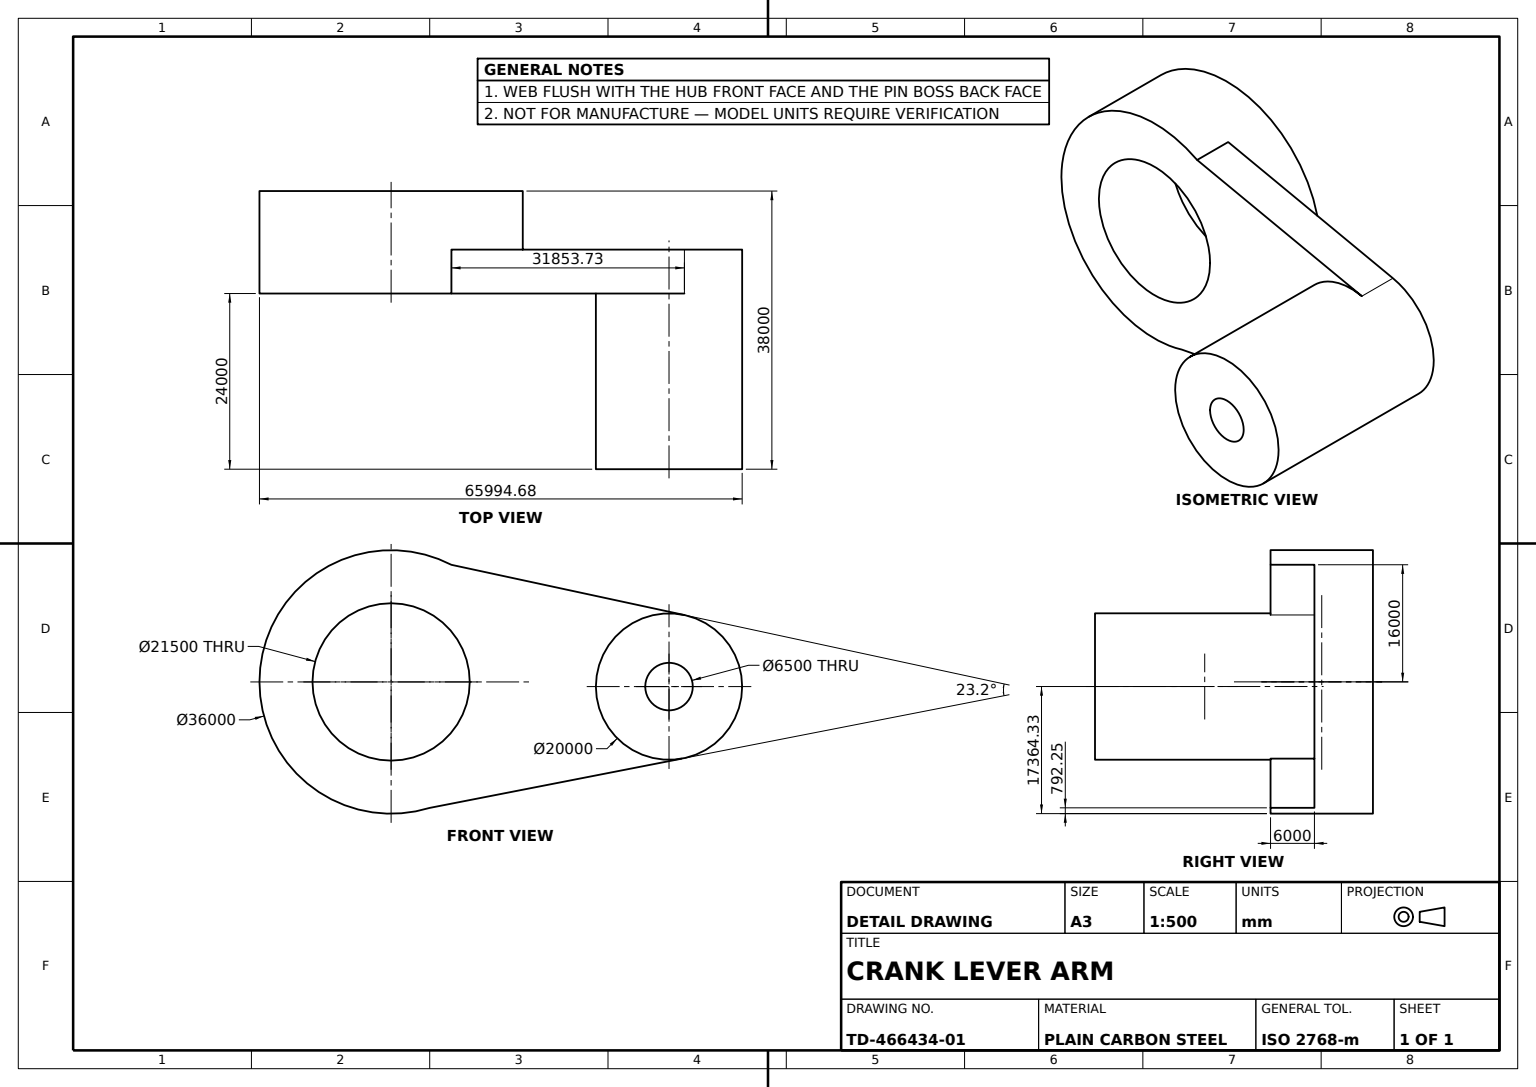
SolidWorks part; units mm, degrees
material "Plain Carbon Steel"
ref_plane "Front Plane" through (0, 0, 0) normal (0, 0, 1) x (1, 0, 0)
ref_plane "Top Plane" through (0, 0, 0) normal (0, 1, 0) x (1, 0, 0)
ref_plane "Right Plane" through (0, 0, 0) normal (1, 0, 0) x (0, 0, -1)
sketch "Main Hub Sketch" plane through (0, 0, 0) normal (0, 0, 1) x (1, 0, 0)
  circle A0 centre (0, 0) radius 18000
  dimension "D1" = 36000
extrude "Main Hub Ø36" add sketch "Main Hub Sketch" against normal blind 14000
sketch "Hub Bore Sketch" plane through (0, 0, -14000) normal (0, 0, -1) x (-1, 0, 0)
  circle A0 centre (0, 0) radius 10750
  dimension "D1" = 21500
extrude "Hub Bore Ø21.5" cut sketch "Hub Bore Sketch" against normal blind 14000
sketch "Arm Web Sketch" plane through (0, 0, 0) normal (0, 0, 1) x (1, 0, 0)
  line L1 (8246.2113, 16000) -> (40099.946, 9140.2103)
  line L3 (5281.4009, -17207.7542) -> (40099.946, -10411.5535)
  arc A0 (40099.946, -10411.5535) -> (40099.946, 9140.2103) centre (37994.6828, -635.6716) ccw
  circle A1 centre (0, 0) radius 18000 construction
  arc A2 (5281.4009, -17207.7542) -> (8246.2113, 16000) centre (0, 0) ccw
  dimension "D1" = 20000
  dimension "D2" = 38000
  dimension "D3" = 34818.5451
  dimension "D4" = 31853.7347
  dimension "D5" = 16000
extrude "Arm Web" add sketch "Arm Web Sketch" against normal blind 6000
sketch "Pin Boss Sketch" plane through (0, 0, 0) normal (0, 0, 1) x (1, 0, 0)
  circle A0 centre (37994.6828, -635.6716) radius 10000
  dimension "D1" = 20000
extrude "Pin Boss Ø20" add sketch "Pin Boss Sketch" along normal blind 24000 and the other way blind 6000
sketch "Pin Hole Sketch" plane through (0, 0, 24000) normal (0, 0, 1) x (1, 0, 0)
  circle A0 centre (37994.6828, -635.6716) radius 3250
  dimension "D1" = 6500
extrude "Pin Hole Ø6.5" cut sketch "Pin Hole Sketch" against normal through all
